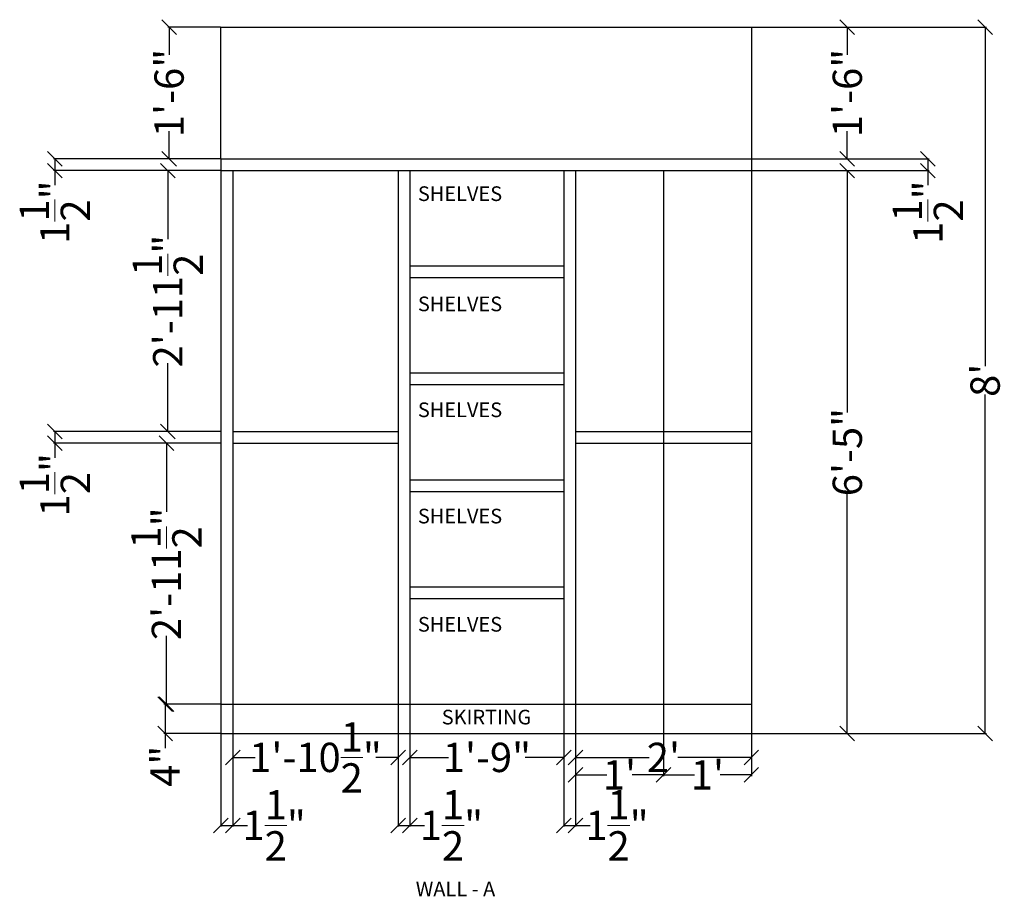
# Model space of a CAD drawing. Units: inches. Extents: x 2723 to 2858, y 1725 to 1845.
import ezdxf

# ---------------------------------------------------------------- set-up
doc = ezdxf.new("R2010")
doc.units = ezdxf.units.IN
doc.header["$MEASUREMENT"] = 0
for name, color, linetype, lineweight in [('A-ANNO-DIMS', 2, 'Continuous', 18), ('A-ANNO-TEXT', 3, 'Continuous', 18), ('A-FURN', 7, 'Continuous', 25)]:
    doc.layers.add(name, color=color, linetype=linetype, lineweight=lineweight)
doc.styles.get("Standard").update_dxf_attribs({"font": 'arial.ttf'})
doc.dimstyles.get("Standard").update_dxf_attribs({"dimtxt": 4, "dimasz": 2, "dimexe": 0.18, "dimexo": 0.0625, "dimgap": 0.09, "dimtad": 0, "dimdec": 1, "dimzin": 0, "dimdsep": 46, "dimlunit": 4, "dimtxsty": 'Standard', "dimblk": 'OBLIQUE', "dimcen": 0.09, "dimadec": 0, "dimazin": 0, "dimtfac": 1, "dimtdec": 1, "dimtofl": 0, "dimtmove": 0, "dimatfit": 3, "dimldrblk": 'OBLIQUE', "dimfxl": 1, "dimtolj": 1, "dimtzin": 0, "dimarcsym": 1})

# ---------------------------------------------------------------- blocks, each defined once
blk = doc.blocks.new('_Oblique')
at = {"color": 0, "linetype": 'ByBlock', "lineweight": -2}
blk.add_line((-0.5, -0.5), (0.5, 0.5), dxfattribs=at)
blk = doc.blocks.new('*D2')
at = {"layer": 'A-ANNO-DIMS', "color": 0, "lineweight": -2, "transparency": 16777216}
for p, q in [((2750.55, 1843.92), (2743.34, 1843.92)), ((2743.52, 1843.92), (2743.52, 1840.14)), ((2743.52, 1825.92), (2743.52, 1829.7)), ((2750.55, 1825.92), (2743.34, 1825.92))]:
    blk.add_line(p, q, dxfattribs=at)
at = {"layer": 'Defpoints', "color": 0, "transparency": 16777216}
for p in [(2743.52, 1843.92), (2750.61, 1843.92), (2750.61, 1825.92)]:
    blk.add_point(p, dxfattribs=at)
at = {"layer": 'A-ANNO-DIMS', "color": 0, "lineweight": -2, "transparency": 16777216, "xscale": 2, "yscale": 2, "zscale": 2}
for p, rotation in [((2743.52, 1843.92), 90), ((2743.52, 1825.92), 270)]:
    blk.add_blockref('_Oblique', p, dxfattribs=dict(at, rotation=rotation))
at = {"layer": 'A-ANNO-DIMS', "color": 0, "transparency": 16777216, "insert": (2743.52, 1834.92), "char_height": 4, "attachment_point": 5, "rotation": 90}
blk.add_mtext('\\A1;1\'-6"', dxfattribs=at)
blk = doc.blocks.new('*D3')
at = {"layer": 'A-ANNO-DIMS', "color": 0, "lineweight": -2, "transparency": 16777216}
for p, q in [((2750.55, 1825.92), (2727.75, 1825.92)), ((2727.93, 1825.92), (2727.93, 1824.32)), ((2750.55, 1824.32), (2727.75, 1824.32)), ((2727.93, 1824.32), (2727.93, 1822.32))]:
    blk.add_line(p, q, dxfattribs=at)
at = {"layer": 'Defpoints', "color": 0, "transparency": 16777216}
for p in [(2750.61, 1825.92), (2727.93, 1824.32), (2750.61, 1824.32)]:
    blk.add_point(p, dxfattribs=at)
at = {"layer": 'A-ANNO-DIMS', "color": 0, "lineweight": -2, "transparency": 16777216, "xscale": 2, "yscale": 2, "zscale": 2}
for p, rotation in [((2727.93, 1825.92), 90), ((2727.93, 1824.32), 270)]:
    blk.add_blockref('_Oblique', p, dxfattribs=dict(at, rotation=rotation))
at = {"layer": 'A-ANNO-DIMS', "color": 0, "transparency": 16777216, "insert": (2727.93, 1818.66), "char_height": 4, "attachment_point": 5, "rotation": 90}
blk.add_mtext('\\A1;1{\\H1x;\\S1/2;}"', dxfattribs=at)
blk = doc.blocks.new('*D4')
at = {"layer": 'A-ANNO-DIMS', "color": 0, "lineweight": -2, "transparency": 16777216}
for p, q in [((2750.55, 1824.32), (2743.16, 1824.32)), ((2743.34, 1824.32), (2743.34, 1814.97)), ((2743.34, 1788.72), (2743.34, 1798.07)), ((2750.55, 1788.72), (2743.16, 1788.72))]:
    blk.add_line(p, q, dxfattribs=at)
at = {"layer": 'Defpoints', "color": 0, "transparency": 16777216}
for p in [(2750.61, 1824.32), (2743.34, 1788.72), (2750.61, 1788.72)]:
    blk.add_point(p, dxfattribs=at)
at = {"layer": 'A-ANNO-DIMS', "color": 0, "lineweight": -2, "transparency": 16777216, "xscale": 2, "yscale": 2, "zscale": 2}
for p, rotation in [((2743.34, 1824.32), 90), ((2743.34, 1788.72), 270)]:
    blk.add_blockref('_Oblique', p, dxfattribs=dict(at, rotation=rotation))
at = {"layer": 'A-ANNO-DIMS', "color": 0, "transparency": 16777216, "insert": (2743.34, 1806.52), "char_height": 4, "attachment_point": 5, "rotation": 90}
blk.add_mtext('\\A1;2\'-11{\\H1x;\\S1/2;}"', dxfattribs=at)
blk = doc.blocks.new('*D5')
at = {"layer": 'A-ANNO-DIMS', "color": 0, "lineweight": -2, "transparency": 16777216}
for p, q in [((2750.55, 1788.72), (2727.75, 1788.72)), ((2727.93, 1788.72), (2727.93, 1787.12)), ((2750.55, 1787.12), (2727.75, 1787.12)), ((2727.93, 1787.12), (2727.93, 1785.12))]:
    blk.add_line(p, q, dxfattribs=at)
at = {"layer": 'Defpoints', "color": 0, "transparency": 16777216}
for p in [(2750.61, 1788.72), (2727.93, 1787.12), (2750.61, 1787.12)]:
    blk.add_point(p, dxfattribs=at)
at = {"layer": 'A-ANNO-DIMS', "color": 0, "lineweight": -2, "transparency": 16777216, "xscale": 2, "yscale": 2, "zscale": 2}
for p, rotation in [((2727.93, 1788.72), 90), ((2727.93, 1787.12), 270)]:
    blk.add_blockref('_Oblique', p, dxfattribs=dict(at, rotation=rotation))
at = {"layer": 'A-ANNO-DIMS', "color": 0, "transparency": 16777216, "insert": (2727.93, 1781.46), "char_height": 4, "attachment_point": 5, "rotation": 90}
blk.add_mtext('\\A1;1{\\H1x;\\S1/2;}"', dxfattribs=at)
blk = doc.blocks.new('*D6')
at = {"layer": 'A-ANNO-DIMS', "color": 0, "lineweight": -2, "transparency": 16777216}
for p, q in [((2750.55, 1787.12), (2742.98, 1787.12)), ((2743.16, 1787.12), (2743.16, 1777.77)), ((2743.16, 1751.52), (2743.16, 1760.87)), ((2750.55, 1751.52), (2742.98, 1751.52))]:
    blk.add_line(p, q, dxfattribs=at)
at = {"layer": 'Defpoints', "color": 0, "transparency": 16777216}
for p in [(2750.61, 1787.12), (2743.16, 1751.52), (2750.61, 1751.52)]:
    blk.add_point(p, dxfattribs=at)
at = {"layer": 'A-ANNO-DIMS', "color": 0, "lineweight": -2, "transparency": 16777216, "xscale": 2, "yscale": 2, "zscale": 2}
for p, rotation in [((2743.16, 1787.12), 90), ((2743.16, 1751.52), 270)]:
    blk.add_blockref('_Oblique', p, dxfattribs=dict(at, rotation=rotation))
at = {"layer": 'A-ANNO-DIMS', "color": 0, "transparency": 16777216, "insert": (2743.16, 1769.32), "char_height": 4, "attachment_point": 5, "rotation": 90}
blk.add_mtext('\\A1;2\'-11{\\H1x;\\S1/2;}"', dxfattribs=at)
blk = doc.blocks.new('*D7')
at = {"layer": 'A-ANNO-DIMS', "color": 0, "lineweight": -2, "transparency": 16777216}
for p, q in [((2750.55, 1751.52), (2742.8, 1751.52)), ((2742.98, 1751.52), (2742.98, 1747.52)), ((2750.55, 1747.52), (2742.8, 1747.52)), ((2742.98, 1747.52), (2742.98, 1745.52))]:
    blk.add_line(p, q, dxfattribs=at)
at = {"layer": 'Defpoints', "color": 0, "transparency": 16777216}
for p in [(2750.61, 1751.52), (2742.98, 1747.52), (2750.61, 1747.52)]:
    blk.add_point(p, dxfattribs=at)
at = {"layer": 'A-ANNO-DIMS', "color": 0, "lineweight": -2, "transparency": 16777216, "xscale": 2, "yscale": 2, "zscale": 2}
for p, rotation in [((2742.98, 1751.52), 90), ((2742.98, 1747.52), 270)]:
    blk.add_blockref('_Oblique', p, dxfattribs=dict(at, rotation=rotation))
at = {"layer": 'A-ANNO-DIMS', "color": 0, "transparency": 16777216, "insert": (2742.98, 1743.05), "char_height": 4, "attachment_point": 5, "rotation": 90}
blk.add_mtext('\\A1;4"', dxfattribs=at)
blk = doc.blocks.new('*D8')
at = {"layer": 'A-ANNO-DIMS', "color": 0, "lineweight": -2, "transparency": 16777216}
for p, q in [((2823.07, 1824.32), (2836.29, 1824.32)), ((2836.11, 1824.32), (2836.11, 1791.34)), ((2836.11, 1747.52), (2836.11, 1780.5)), ((2823.07, 1747.52), (2836.29, 1747.52))]:
    blk.add_line(p, q, dxfattribs=at)
at = {"layer": 'Defpoints', "color": 0, "transparency": 16777216}
for p in [(2823.01, 1824.32), (2823.01, 1747.52), (2836.11, 1747.52)]:
    blk.add_point(p, dxfattribs=at)
at = {"layer": 'A-ANNO-DIMS', "color": 0, "lineweight": -2, "transparency": 16777216, "xscale": 2, "yscale": 2, "zscale": 2}
for p, rotation in [((2836.11, 1824.32), 90), ((2836.11, 1747.52), 270)]:
    blk.add_blockref('_Oblique', p, dxfattribs=dict(at, rotation=rotation))
at = {"layer": 'A-ANNO-DIMS', "color": 0, "transparency": 16777216, "insert": (2836.11, 1785.92), "char_height": 4, "attachment_point": 5, "rotation": 90}
blk.add_mtext('\\A1;6\'-5"', dxfattribs=at)
blk = doc.blocks.new('*D9')
at = {"layer": 'A-ANNO-DIMS', "color": 0, "lineweight": -2, "transparency": 16777216}
for p, q in [((2823.07, 1843.92), (2836.29, 1843.92)), ((2836.11, 1843.92), (2836.11, 1840.14)), ((2836.11, 1825.92), (2836.11, 1829.7)), ((2823.07, 1825.92), (2836.29, 1825.92))]:
    blk.add_line(p, q, dxfattribs=at)
at = {"layer": 'Defpoints', "color": 0, "transparency": 16777216}
for p in [(2823.01, 1843.92), (2823.01, 1825.92), (2836.11, 1825.92)]:
    blk.add_point(p, dxfattribs=at)
at = {"layer": 'A-ANNO-DIMS', "color": 0, "lineweight": -2, "transparency": 16777216, "xscale": 2, "yscale": 2, "zscale": 2}
for p, rotation in [((2836.11, 1843.92), 90), ((2836.11, 1825.92), 270)]:
    blk.add_blockref('_Oblique', p, dxfattribs=dict(at, rotation=rotation))
at = {"layer": 'A-ANNO-DIMS', "color": 0, "transparency": 16777216, "insert": (2836.11, 1834.92), "char_height": 4, "attachment_point": 5, "rotation": 90}
blk.add_mtext('\\A1;1\'-6"', dxfattribs=at)
blk = doc.blocks.new('*D10')
at = {"layer": 'A-ANNO-DIMS', "color": 0, "lineweight": -2, "transparency": 16777216}
for p, q in [((2823.07, 1825.92), (2847.29, 1825.92)), ((2847.11, 1825.92), (2847.11, 1824.32)), ((2823.07, 1824.32), (2847.29, 1824.32)), ((2847.11, 1824.32), (2847.11, 1822.32))]:
    blk.add_line(p, q, dxfattribs=at)
at = {"layer": 'Defpoints', "color": 0, "transparency": 16777216}
for p in [(2823.01, 1825.92), (2823.01, 1824.32), (2847.11, 1824.32)]:
    blk.add_point(p, dxfattribs=at)
at = {"layer": 'A-ANNO-DIMS', "color": 0, "lineweight": -2, "transparency": 16777216, "xscale": 2, "yscale": 2, "zscale": 2}
for p, rotation in [((2847.11, 1825.92), 90), ((2847.11, 1824.32), 270)]:
    blk.add_blockref('_Oblique', p, dxfattribs=dict(at, rotation=rotation))
at = {"layer": 'A-ANNO-DIMS', "color": 0, "transparency": 16777216, "insert": (2847.11, 1818.66), "char_height": 4, "attachment_point": 5, "rotation": 90}
blk.add_mtext('\\A1;1{\\H1x;\\S1/2;}"', dxfattribs=at)
blk = doc.blocks.new('*D11')
at = {"layer": 'A-ANNO-DIMS', "color": 0, "lineweight": -2, "transparency": 16777216}
for p, q in [((2823.07, 1843.92), (2855.1, 1843.92)), ((2854.92, 1843.92), (2854.92, 1797.65)), ((2854.92, 1747.52), (2854.92, 1793.79)), ((2823.07, 1747.52), (2855.1, 1747.52))]:
    blk.add_line(p, q, dxfattribs=at)
at = {"layer": 'Defpoints', "color": 0, "transparency": 16777216}
for p in [(2823.01, 1843.92), (2823.01, 1747.52), (2854.92, 1747.52)]:
    blk.add_point(p, dxfattribs=at)
at = {"layer": 'A-ANNO-DIMS', "color": 0, "lineweight": -2, "transparency": 16777216, "xscale": 2, "yscale": 2, "zscale": 2}
for p, rotation in [((2854.92, 1843.92), 90), ((2854.92, 1747.52), 270)]:
    blk.add_blockref('_Oblique', p, dxfattribs=dict(at, rotation=rotation))
at = {"layer": 'A-ANNO-DIMS', "color": 0, "transparency": 16777216, "insert": (2854.92, 1795.72), "char_height": 4, "attachment_point": 5, "rotation": 90}
blk.add_mtext("\\A1;8'", dxfattribs=at)
blk = doc.blocks.new('*D12')
at = {"layer": 'A-ANNO-DIMS', "color": 0, "lineweight": -2, "transparency": 16777216}
for p, q in [((2750.61, 1751.46), (2750.61, 1734.81)), ((2752.21, 1751.46), (2752.21, 1734.81)), ((2750.61, 1734.99), (2752.21, 1734.99)), ((2752.21, 1734.99), (2754.21, 1734.99))]:
    blk.add_line(p, q, dxfattribs=at)
at = {"layer": 'Defpoints', "color": 0, "transparency": 16777216}
for p in [(2750.61, 1751.52), (2752.21, 1751.52), (2752.21, 1734.99)]:
    blk.add_point(p, dxfattribs=at)
at = {"layer": 'A-ANNO-DIMS', "color": 0, "lineweight": -2, "transparency": 16777216, "xscale": 2, "yscale": 2, "zscale": 2, "rotation": 180}
blk.add_blockref('_Oblique', (2750.61, 1734.99), dxfattribs=at)
at = {"layer": 'A-ANNO-DIMS', "color": 0, "lineweight": -2, "transparency": 16777216, "xscale": 2, "yscale": 2, "zscale": 2}
blk.add_blockref('_Oblique', (2752.21, 1734.99), dxfattribs=at)
at = {"layer": 'A-ANNO-DIMS', "color": 0, "transparency": 16777216, "insert": (2757.87, 1734.99), "char_height": 4, "attachment_point": 5}
blk.add_mtext('\\A1;1{\\H1x;\\S1/2;}"', dxfattribs=at)
blk = doc.blocks.new('*D13')
at = {"layer": 'A-ANNO-DIMS', "color": 0, "lineweight": -2, "transparency": 16777216}
for p, q in [((2752.21, 1751.46), (2752.21, 1744.08)), ((2774.81, 1751.46), (2774.81, 1744.08)), ((2752.21, 1744.26), (2755.28, 1744.26)), ((2774.81, 1744.26), (2771.74, 1744.26))]:
    blk.add_line(p, q, dxfattribs=at)
at = {"layer": 'Defpoints', "color": 0, "transparency": 16777216}
for p in [(2752.21, 1751.52), (2774.81, 1751.52), (2774.81, 1744.26)]:
    blk.add_point(p, dxfattribs=at)
at = {"layer": 'A-ANNO-DIMS', "color": 0, "lineweight": -2, "transparency": 16777216, "xscale": 2, "yscale": 2, "zscale": 2, "rotation": 180}
blk.add_blockref('_Oblique', (2752.21, 1744.26), dxfattribs=at)
at = {"layer": 'A-ANNO-DIMS', "color": 0, "lineweight": -2, "transparency": 16777216, "xscale": 2, "yscale": 2, "zscale": 2}
blk.add_blockref('_Oblique', (2774.81, 1744.26), dxfattribs=at)
at = {"layer": 'A-ANNO-DIMS', "color": 0, "transparency": 16777216, "insert": (2763.51, 1744.26), "char_height": 4, "attachment_point": 5}
blk.add_mtext('\\A1;1\'-10{\\H1x;\\S1/2;}"', dxfattribs=at)
blk = doc.blocks.new('*D14')
at = {"layer": 'A-ANNO-DIMS', "color": 0, "lineweight": -2, "transparency": 16777216}
for p, q in [((2774.81, 1751.46), (2774.81, 1734.81)), ((2776.41, 1751.46), (2776.41, 1734.81)), ((2774.81, 1734.99), (2776.41, 1734.99)), ((2776.41, 1734.99), (2778.41, 1734.99))]:
    blk.add_line(p, q, dxfattribs=at)
at = {"layer": 'Defpoints', "color": 0, "transparency": 16777216}
for p in [(2774.81, 1751.52), (2776.41, 1751.52), (2776.41, 1734.99)]:
    blk.add_point(p, dxfattribs=at)
at = {"layer": 'A-ANNO-DIMS', "color": 0, "lineweight": -2, "transparency": 16777216, "xscale": 2, "yscale": 2, "zscale": 2, "rotation": 180}
blk.add_blockref('_Oblique', (2774.81, 1734.99), dxfattribs=at)
at = {"layer": 'A-ANNO-DIMS', "color": 0, "lineweight": -2, "transparency": 16777216, "xscale": 2, "yscale": 2, "zscale": 2}
blk.add_blockref('_Oblique', (2776.41, 1734.99), dxfattribs=at)
at = {"layer": 'A-ANNO-DIMS', "color": 0, "transparency": 16777216, "insert": (2782.07, 1734.99), "char_height": 4, "attachment_point": 5}
blk.add_mtext('\\A1;1{\\H1x;\\S1/2;}"', dxfattribs=at)
blk = doc.blocks.new('*D15')
at = {"layer": 'A-ANNO-DIMS', "color": 0, "lineweight": -2, "transparency": 16777216}
for p, q in [((2776.41, 1751.46), (2776.41, 1744.08)), ((2797.41, 1751.46), (2797.41, 1744.08)), ((2776.41, 1744.26), (2781.69, 1744.26)), ((2797.41, 1744.26), (2792.13, 1744.26))]:
    blk.add_line(p, q, dxfattribs=at)
at = {"layer": 'Defpoints', "color": 0, "transparency": 16777216}
for p in [(2776.41, 1751.52), (2797.41, 1751.52), (2797.41, 1744.26)]:
    blk.add_point(p, dxfattribs=at)
at = {"layer": 'A-ANNO-DIMS', "color": 0, "lineweight": -2, "transparency": 16777216, "xscale": 2, "yscale": 2, "zscale": 2, "rotation": 180}
blk.add_blockref('_Oblique', (2776.41, 1744.26), dxfattribs=at)
at = {"layer": 'A-ANNO-DIMS', "color": 0, "lineweight": -2, "transparency": 16777216, "xscale": 2, "yscale": 2, "zscale": 2}
blk.add_blockref('_Oblique', (2797.41, 1744.26), dxfattribs=at)
at = {"layer": 'A-ANNO-DIMS', "color": 0, "transparency": 16777216, "insert": (2786.91, 1744.26), "char_height": 4, "attachment_point": 5}
blk.add_mtext('\\A1;1\'-9"', dxfattribs=at)
blk = doc.blocks.new('*D16')
at = {"layer": 'A-ANNO-DIMS', "color": 0, "lineweight": -2, "transparency": 16777216}
for p, q in [((2797.41, 1751.46), (2797.41, 1734.81)), ((2799.01, 1751.46), (2799.01, 1734.81)), ((2797.41, 1734.99), (2799.01, 1734.99)), ((2799.01, 1734.99), (2801.01, 1734.99))]:
    blk.add_line(p, q, dxfattribs=at)
at = {"layer": 'Defpoints', "color": 0, "transparency": 16777216}
for p in [(2797.41, 1751.52), (2799.01, 1751.52), (2799.01, 1734.99)]:
    blk.add_point(p, dxfattribs=at)
at = {"layer": 'A-ANNO-DIMS', "color": 0, "lineweight": -2, "transparency": 16777216, "xscale": 2, "yscale": 2, "zscale": 2, "rotation": 180}
blk.add_blockref('_Oblique', (2797.41, 1734.99), dxfattribs=at)
at = {"layer": 'A-ANNO-DIMS', "color": 0, "lineweight": -2, "transparency": 16777216, "xscale": 2, "yscale": 2, "zscale": 2}
blk.add_blockref('_Oblique', (2799.01, 1734.99), dxfattribs=at)
at = {"layer": 'A-ANNO-DIMS', "color": 0, "transparency": 16777216, "insert": (2804.67, 1734.99), "char_height": 4, "attachment_point": 5}
blk.add_mtext('\\A1;1{\\H1x;\\S1/2;}"', dxfattribs=at)
blk = doc.blocks.new('*D17')
at = {"layer": 'A-ANNO-DIMS', "color": 0, "lineweight": -2, "transparency": 16777216}
for p, q in [((2799.01, 1751.46), (2799.01, 1744.08)), ((2823.01, 1751.46), (2823.01, 1744.08)), ((2799.01, 1744.26), (2809.04, 1744.26)), ((2823.01, 1744.26), (2812.97, 1744.26))]:
    blk.add_line(p, q, dxfattribs=at)
at = {"layer": 'Defpoints', "color": 0, "transparency": 16777216}
for p in [(2799.01, 1751.52), (2823.01, 1751.52), (2823.01, 1744.26)]:
    blk.add_point(p, dxfattribs=at)
at = {"layer": 'A-ANNO-DIMS', "color": 0, "lineweight": -2, "transparency": 16777216, "xscale": 2, "yscale": 2, "zscale": 2, "rotation": 180}
blk.add_blockref('_Oblique', (2799.01, 1744.26), dxfattribs=at)
at = {"layer": 'A-ANNO-DIMS', "color": 0, "lineweight": -2, "transparency": 16777216, "xscale": 2, "yscale": 2, "zscale": 2}
blk.add_blockref('_Oblique', (2823.01, 1744.26), dxfattribs=at)
at = {"layer": 'A-ANNO-DIMS', "color": 0, "transparency": 16777216, "insert": (2811.01, 1744.26), "char_height": 4, "attachment_point": 5}
blk.add_mtext("\\A1;2'", dxfattribs=at)
blk = doc.blocks.new('*D18')
at = {"layer": 'A-ANNO-DIMS', "color": 0, "lineweight": -2, "transparency": 16777216}
for p, q in [((2799.01, 1751.46), (2799.01, 1741.7)), ((2811.01, 1751.46), (2811.01, 1741.7)), ((2799.01, 1741.88), (2803.27, 1741.88)), ((2811.01, 1741.88), (2806.75, 1741.88))]:
    blk.add_line(p, q, dxfattribs=at)
at = {"layer": 'Defpoints', "color": 0, "transparency": 16777216}
for p in [(2799.01, 1751.52), (2811.01, 1751.52), (2811.01, 1741.88)]:
    blk.add_point(p, dxfattribs=at)
at = {"layer": 'A-ANNO-DIMS', "color": 0, "lineweight": -2, "transparency": 16777216, "xscale": 2, "yscale": 2, "zscale": 2, "rotation": 180}
blk.add_blockref('_Oblique', (2799.01, 1741.88), dxfattribs=at)
at = {"layer": 'A-ANNO-DIMS', "color": 0, "lineweight": -2, "transparency": 16777216, "xscale": 2, "yscale": 2, "zscale": 2}
blk.add_blockref('_Oblique', (2811.01, 1741.88), dxfattribs=at)
at = {"layer": 'A-ANNO-DIMS', "color": 0, "transparency": 16777216, "insert": (2805.01, 1741.88), "char_height": 4, "attachment_point": 5}
blk.add_mtext("\\A1;1'", dxfattribs=at)
blk = doc.blocks.new('*D19')
at = {"layer": 'A-ANNO-DIMS', "color": 0, "lineweight": -2, "transparency": 16777216}
for p, q in [((2811.01, 1751.46), (2811.01, 1741.7)), ((2823.01, 1751.46), (2823.01, 1741.7)), ((2811.01, 1741.88), (2815.27, 1741.88)), ((2823.01, 1741.88), (2818.75, 1741.88))]:
    blk.add_line(p, q, dxfattribs=at)
at = {"layer": 'Defpoints', "color": 0, "transparency": 16777216}
for p in [(2811.01, 1751.52), (2823.01, 1751.52), (2823.01, 1741.88)]:
    blk.add_point(p, dxfattribs=at)
at = {"layer": 'A-ANNO-DIMS', "color": 0, "lineweight": -2, "transparency": 16777216, "xscale": 2, "yscale": 2, "zscale": 2, "rotation": 180}
blk.add_blockref('_Oblique', (2811.01, 1741.88), dxfattribs=at)
at = {"layer": 'A-ANNO-DIMS', "color": 0, "lineweight": -2, "transparency": 16777216, "xscale": 2, "yscale": 2, "zscale": 2}
blk.add_blockref('_Oblique', (2823.01, 1741.88), dxfattribs=at)
at = {"layer": 'A-ANNO-DIMS', "color": 0, "transparency": 16777216, "insert": (2817.01, 1741.88), "char_height": 4, "attachment_point": 5}
blk.add_mtext("\\A1;1'", dxfattribs=at)

msp = doc.modelspace()

# ---------------------------------------------------------------- linework, layer by layer
at = {"layer": 'A-FURN'}
for p, q in [((2750.61, 1825.92), (2750.61, 1843.92)), ((2750.61, 1843.92), (2823.01, 1843.92)), ((2823.01, 1843.92), (2823.01, 1747.52)), ((2750.61, 1825.92), (2752.21, 1825.92)), ((2750.61, 1825.92), (2750.61, 1824.32)), ((2752.21, 1825.92), (2774.81, 1825.92)), ((2774.81, 1825.92), (2776.41, 1825.92)), ((2776.41, 1825.92), (2797.41, 1825.92)), ((2797.41, 1825.92), (2799.01, 1825.92)), ((2799.01, 1825.92), (2823.01, 1825.92)), ((2750.61, 1824.32), (2750.61, 1788.72)), ((2750.61, 1824.32), (2774.81, 1824.32)), ((2752.21, 1824.32), (2752.21, 1751.52)), ((2774.81, 1824.32), (2774.81, 1751.52)), ((2774.81, 1824.32), (2799.01, 1824.32)), ((2776.41, 1824.32), (2776.41, 1751.52)), ((2797.41, 1824.32), (2797.41, 1751.52)), ((2799.01, 1824.32), (2799.01, 1751.52)), ((2799.01, 1824.32), (2823.01, 1824.32)), ((2811.01, 1824.32), (2811.01, 1751.52)), ((2776.41, 1811.32), (2797.41, 1811.32)), ((2776.41, 1809.72), (2797.41, 1809.72)), ((2776.41, 1796.72), (2797.41, 1796.72)), ((2776.41, 1795.12), (2797.41, 1795.12)), ((2750.61, 1788.72), (2750.61, 1787.12)), ((2752.21, 1788.72), (2774.81, 1788.72)), ((2799.01, 1788.72), (2823.01, 1788.72)), ((2750.61, 1787.12), (2750.61, 1751.52)), ((2752.21, 1787.12), (2774.81, 1787.12)), ((2799.01, 1787.12), (2823.01, 1787.12)), ((2776.41, 1782.12), (2797.41, 1782.12)), ((2776.41, 1780.52), (2797.41, 1780.52)), ((2776.41, 1767.52), (2797.41, 1767.52)), ((2776.41, 1765.92), (2797.41, 1765.92)), ((2750.61, 1751.52), (2750.61, 1747.52)), ((2750.61, 1751.52), (2823.01, 1751.52)), ((2750.61, 1747.52), (2823.01, 1747.52))]:
    msp.add_line(p, q, dxfattribs=at)

# ---------------------------------------------------------------- texts
at = {"layer": 'A-ANNO-TEXT', "char_height": 2, "attachment_point": 1}
for s, width, heights, insert in [('SHELVES', 12.882, [2.07], (2777.49, 1822.18)), ('SHELVES', 12.882, [2.07], (2777.49, 1807.14)), ('SHELVES', 12.882, [2.07], (2777.49, 1792.69)), ('SHELVES', 12.882, [2.07], (2777.49, 1778.19)), ('SHELVES', 12.882, [2.07], (2777.49, 1763.42)), ('\\pxqc;SKIRTING', 16.1643, [0], (2778.77, 1750.76)), ('\\pxqc;WALL - A', 67.0442, [0], (2749.1, 1727.31))]:
    msp.add_mtext_dynamic_manual_height_columns(s, width=width, gutter_width=10, heights=heights, dxfattribs=dict(at, insert=insert))

# ---------------------------------------------------------------- dimensions: what is measured, and where the dimension line sits
at = {"layer": 'A-ANNO-DIMS'}
for base, p1, p2, picture, middle in [((2743.52, 1843.92), (2750.61, 1825.92), (2750.61, 1843.92), '*D2', (2743.52, 1834.92)), ((2836.11, 1825.92), (2823.01, 1843.92), (2823.01, 1825.92), '*D9', (2836.11, 1834.92)), ((2727.93, 1824.32), (2750.61, 1825.92), (2750.61, 1824.32), '*D3', (2727.93, 1818.66)), ((2847.11, 1824.32), (2823.01, 1825.92), (2823.01, 1824.32), '*D10', (2847.11, 1818.66)), ((2743.34, 1788.72), (2750.61, 1824.32), (2750.61, 1788.72), '*D4', (2743.34, 1806.52)), ((2836.11, 1747.52), (2823.01, 1824.32), (2823.01, 1747.52), '*D8', (2836.11, 1785.92)), ((2727.93, 1787.12), (2750.61, 1788.72), (2750.61, 1787.12), '*D5', (2727.93, 1781.46)), ((2743.16, 1751.52), (2750.61, 1787.12), (2750.61, 1751.52), '*D6', (2743.16, 1769.32)), ((2742.98, 1747.52), (2750.61, 1751.52), (2750.61, 1747.52), '*D7', (2742.98, 1743.05))]:
    dim = msp.add_linear_dim(base=base, p1=p1, p2=p2, angle=90, dimstyle='Standard', override={"dimclrd": 0, "dimclre": 0, "dimclrt": 0}, dxfattribs=at)
    dim.commit()
    dim.dimension.update_dxf_attribs({"geometry": picture, "text_midpoint": middle})
dim = msp.add_linear_dim(base=(2854.92, 1747.52), p1=(2823.01, 1843.92), p2=(2823.01, 1747.52), angle=90, text="8'", dimstyle='Standard', override={"dimclrd": 0, "dimclre": 0, "dimclrt": 0}, dxfattribs=at)
dim.commit()
dim.dimension.update_dxf_attribs({"geometry": '*D11', "text_midpoint": (2854.92, 1795.72)})
for base, p1, p2, picture, middle in [((2752.21, 1734.99), (2750.61, 1751.52), (2752.21, 1751.52), '*D12', (2757.87, 1734.99)), ((2774.81, 1744.26), (2752.21, 1751.52), (2774.81, 1751.52), '*D13', (2763.51, 1744.26)), ((2776.41, 1734.99), (2774.81, 1751.52), (2776.41, 1751.52), '*D14', (2782.07, 1734.99)), ((2797.41, 1744.26), (2776.41, 1751.52), (2797.41, 1751.52), '*D15', (2786.91, 1744.26)), ((2799.01, 1734.99), (2797.41, 1751.52), (2799.01, 1751.52), '*D16', (2804.67, 1734.99)), ((2823.01, 1744.26), (2799.01, 1751.52), (2823.01, 1751.52), '*D17', (2811.01, 1744.26)), ((2811.01, 1741.88), (2799.01, 1751.52), (2811.01, 1751.52), '*D18', (2805.01, 1741.88)), ((2823.01, 1741.88), (2811.01, 1751.52), (2823.01, 1751.52), '*D19', (2817.01, 1741.88))]:
    dim = msp.add_linear_dim(base=base, p1=p1, p2=p2, dimstyle='Standard', override={"dimclrd": 0, "dimclre": 0, "dimclrt": 0}, dxfattribs=at)
    dim.commit()
    dim.dimension.update_dxf_attribs({"geometry": picture, "text_midpoint": middle})

doc.saveas('drawing.dxf')
